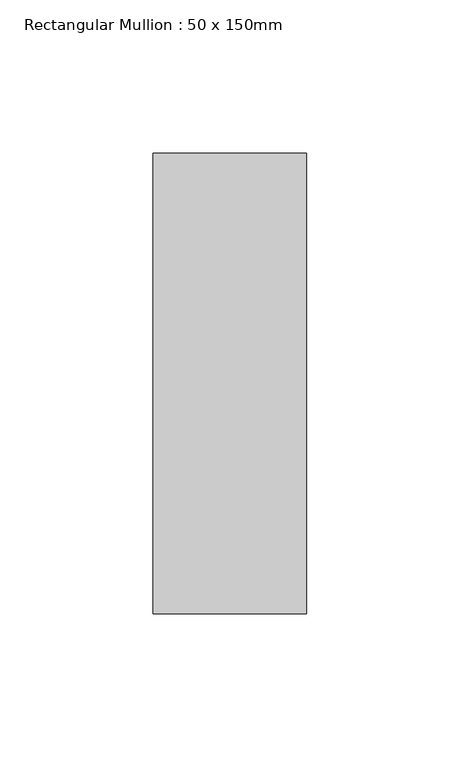
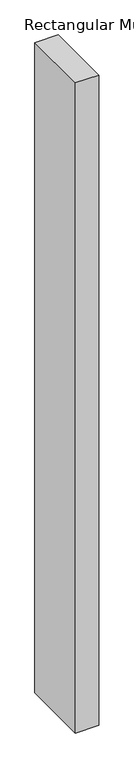
"""IFC4 building model written with IfcOpenShell, lengths in millimetres: member geometry, Rectangular Mullion : 50 x 150mm."""

from ifc_helpers import new_model, si_unit, frame, origin, place, context, project, spatial, polyline, outline, extrude, source, transform, mapped, element, save


def rectangular_mullion_50_x_150mm_59b4522d(model_context):
    return source(origin(), model_context, "Body", "SweptSolid", [
        extrude(outline(polyline([(25.0, 75.0), (25.0, -75.0), (-25.0, -75.0), (-25.0, 75.0), (25.0, 75.0)])), frame((0.0, 0.0, -1466.6666665), z_axis=(0.0, 0.0, 1.0), x_axis=(1.0, 0.0, 0.0)), (0.0, 0.0, 1.0), 1466.6666665),
    ])


if __name__ == "__main__":
    model = new_model("IFC4")
    model_context = context("Model", 3, world=origin())
    ifc_project = project(units=[si_unit("LENGTHUNIT", "METRE", prefix="MILLI")], contexts=[model_context])
    site = spatial("IfcSite", under=ifc_project)
    building = spatial("IfcBuilding", under=site)
    placement = place(None, origin())
    rectangular_mullion_50_x_150mm_shape = rectangular_mullion_50_x_150mm_59b4522d(model_context)
    element("IfcMember", 1, ObjectType="Rectangular Mullion : 50 x 150mm", at=placement, inside=building, context=model_context, shape_type="MappedRepresentation", body=[
        mapped(rectangular_mullion_50_x_150mm_shape, transform((0.0, 0.0, 0.0), x_axis=(1.0, 0.0, 0.0), y_axis=(0.0, 1.0, 0.0), z_axis=(0.0, 0.0, 1.0))),
    ])
    save(model, "model.ifc")

# Revit data of these elements
# Type "Rectangular Mullion : 50 x 150mm"
#   built-in parameter 1007304 = 0.492126 (stored number, unit not read)
#   built-in parameter 1007301 = 0.082021 (stored number, unit not read)
#   built-in parameter 1007300 = 0.082021 (stored number, unit not read)
# Element 1 (IfcMember, "Rectangular Mullion : 50 x 150mm")
#   Materials on its faces: "Aluminium"
# Materials
#   "Aluminium": class "Metal", colour RGB 247 247 247, transparency 0, Description = "Aluminium 6061", Cost = 0
